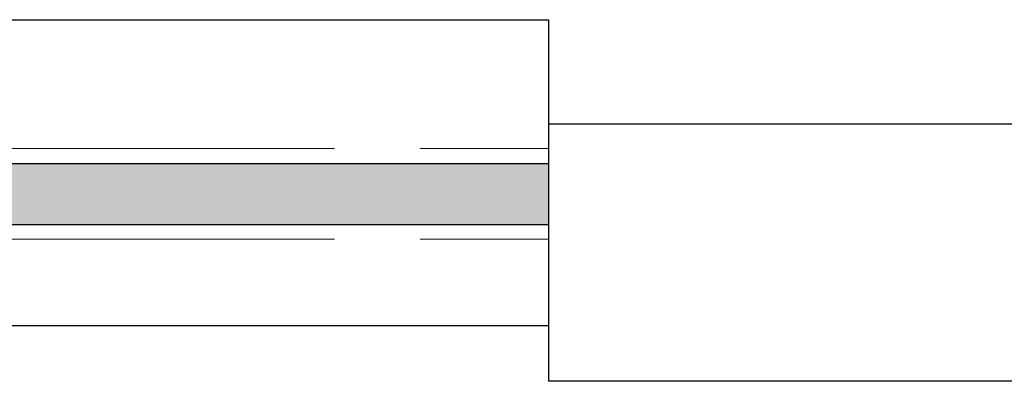
# Model space of a CAD drawing. Units: millimetres. Extents: x 595116 to 630915, y 909473 to 920225.
# Tile 94 of 134: x 629791 to 629825, y 919142 to 919155. Entities that reach past the tile are written whole.
import ezdxf

# ---------------------------------------------------------------- set-up
doc = ezdxf.new("R2010")
doc.units = ezdxf.units.MM
doc.linetypes.add('ACAD_ISO02W100', pattern=[15, 12, -3])
doc.layers.add('C-PROP', color=7, linetype='Continuous', lineweight=25)
doc.layers.add('C-PROP-REF', color=240, linetype='ACAD_ISO02W100', lineweight=13)

msp = doc.modelspace()

# ---------------------------------------------------------------- hatches: boundary and pattern name
at = {"layer": 'C-PROP'}
h = msp.add_hatch(color=256, dxfattribs=at)
h.dxf.hatch_style = 1
h.paths.add_polyline_path([(629809.541, 919149.555), (629625.041, 919149.555), (629625.041, 919147.413), (629809.541, 919147.413)])

# ---------------------------------------------------------------- linework, layer by layer
for p, q in [((629833.541, 919150.928), (629809.541, 919150.928)), ((629809.541, 919150.928), (629809.541, 919141.928)), ((629625.041, 919149.555), (629809.541, 919149.555)), ((629625.041, 919147.413), (629809.541, 919147.413))]:
    msp.add_line(p, q, dxfattribs=at)
msp.add_lwpolyline([(629809.541, 919143.864), (629625.041, 919143.864), (629625.041, 919154.587), (629809.541, 919154.587)], close=True, dxfattribs=at)
msp.add_lwpolyline([(629842.541, 919141.928), (629809.541, 919141.928)], dxfattribs=at)
at = {"layer": 'C-PROP-REF'}
for p, q in [((629625.041, 919150.076), (629809.541, 919150.076)), ((629625.041, 919146.905), (629809.541, 919146.905))]:
    msp.add_line(p, q, dxfattribs=at)

doc.saveas('drawing.dxf')
